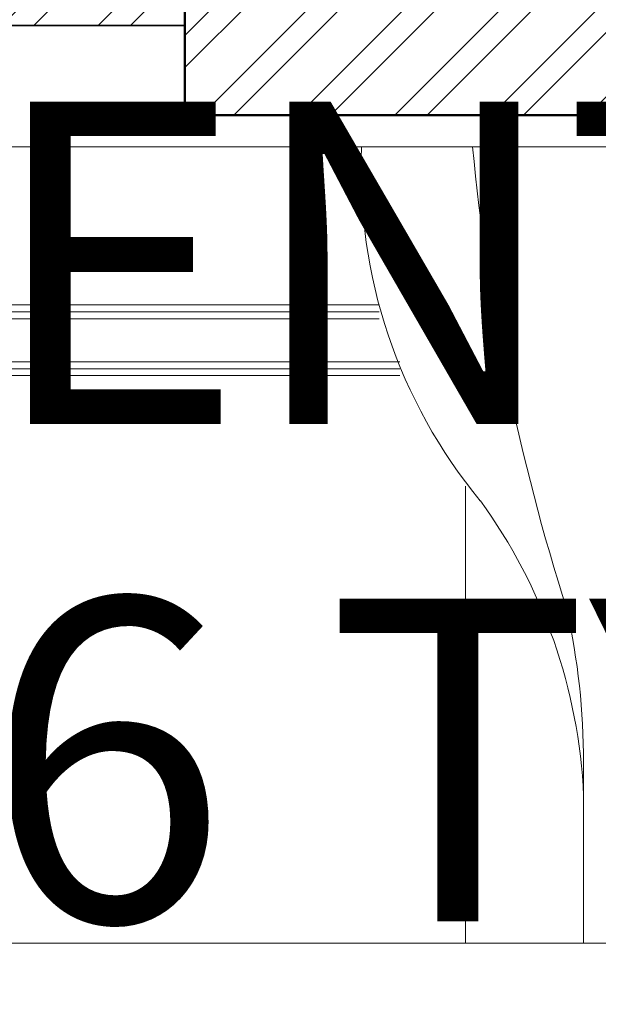
# Model space of a CAD drawing. Units: inches. Extents: x -90 to 536, y -553 to 299.
# Tile 8 of 27: x 122 to 155, y -394 to -339. Entities that reach past the tile are written whole.
import ezdxf

# ---------------------------------------------------------------- set-up
doc = ezdxf.new("R2010")
doc.units = ezdxf.units.IN
for name, color, linetype, lineweight in [('A-ANNO-DIMS', 2, 'Continuous', 18), ('A-DOOR', 4, 'Continuous', 25), ('A-WALL-PATT', 252, 'Continuous', 13), ('Furniture', 2, 'Continuous', 18), ('Inner Wall', 5, 'Continuous', 35), ('Outer Wall', 1, 'Continuous', 50)]:
    doc.layers.add(name, color=color, linetype=linetype, lineweight=lineweight)
doc.styles.get("Standard").update_dxf_attribs({"font": 'arial.ttf'})
doc.dimstyles.get("Standard").update_dxf_attribs({"dimtxt": 18, "dimasz": 12, "dimexe": 0.18, "dimexo": 0.0625, "dimgap": 0.09, "dimtad": 0, "dimtih": 1, "dimtoh": 1, "dimdec": 0, "dimzin": 0, "dimdsep": 46, "dimlunit": 3, "dimtxsty": 'Standard', "dimcen": 0.09, "dimadec": 0, "dimazin": 0, "dimtfac": 1, "dimtdec": 0, "dimtofl": 0, "dimtmove": 0, "dimatfit": 3, "dimfxl": 1, "dimtolj": 1, "dimtzin": 0, "dimarcsym": 0})

# ---------------------------------------------------------------- blocks, each defined once
blk = doc.blocks.new('A$C62731D1C')
for p, q in [((0.0963, 0.3882, 0.6857), (0.0963, 2.1408, 0.6857)), ((1.4679, 2.1408, 0.6857), (1.4679, 0.3882, 0.6857)), ((1.1569, 1.7598, 0.6857), (1.4679, 1.7598, 0.6857)), ((0.6805, 1.5566, 0.6857), (1.4679, 1.5566, 0.6857)), ((0.4664, 1.4437, 0.6857), (0.4664, 0.312, 0.6857)), ((0.4784, 1.4437, 0.6857), (0.4784, 0.312, 0.6857)), ((0.4904, 1.4437, 0.6857), (0.4904, 0.312, 0.6857)), ((0.3683, 1.4076, 0.6857), (0.3683, 0.312, 0.6857)), ((0.3803, 1.4076, 0.6857), (0.3803, 0.312, 0.6857)), ((0.3923, 1.4076, 0.6857), (0.3923, 0.312, 0.6857))]:
    blk.add_line(p, q)
for centre, radius, start, end in [((1.2552, 0.827, 0.6857), 0.9338, 92.5398, 126.0403), ((1.1565, 0.5405, 0.6857), 1.2193, 89.9814, 102.4667), ((-0.2581, 5.3461, 0.6857), 3.7939, 275.3572, 287.6665), ((0.1344, 2.2742, 0.6857), 0.8976, 267.5673, 309.5461)]:
    blk.add_arc(centre, radius, start, end)
blk = doc.blocks.new('A$C0E6D7E3D')
blk.add_blockref('A$C62731D1C', (0, 0))
blk = doc.blocks.new('DOOR-36-B')
for points in [[(37.5, 36), (37.5, 34.5), (36, 34.5), (36, 35.25), (34.5, 35.25), (34.5, 36)], [(0, 0.75), (0, 1.5), (34.5, 1.5), (34.5, 0.75)], [(37.5, 0), (37.5, 1.5), (36, 1.5), (36, 0.75), (34.5, 0.75), (34.5, 0)]]:
    blk.add_lwpolyline(points, close=True)
blk.add_arc((33.758, 1.5), 33.758, 88.7408, 180)
blk = doc.blocks.new('*D27')
at = {"layer": 'A-ANNO-DIMS', "color": 0, "lineweight": -2, "transparency": 16777216}
for p, q in [((49.132, -428.616), (49.132, -434.359)), ((86.632, -428.616), (86.632, -434.359)), ((61.132, -434.179), (74.632, -434.179)), ((86.632, -434.179), (98.632, -434.179))]:
    blk.add_line(p, q, dxfattribs=at)
at = {"layer": 'A-ANNO-DIMS', "color": 0, "transparency": 16777216}
for points in [[(61.132, -432.179), (61.132, -436.179), (49.132, -434.179)], [(74.632, -432.179), (74.632, -436.179), (86.632, -434.179)]]:
    blk.add_solid(points, dxfattribs=at)
at = {"layer": 'Defpoints', "color": 0, "transparency": 16777216}
for p in [(49.132, -428.554), (86.632, -428.554), (86.632, -434.179)]:
    blk.add_point(p, dxfattribs=at)
at = {"layer": 'A-ANNO-DIMS', "color": 0, "transparency": 16777216, "insert": (195.174, -434.179), "char_height": 18, "attachment_point": 5}
blk.add_mtext('\\A1;DOOR B 38 TYP.', dxfattribs=at)
blk = doc.blocks.new('*D28')
at = {"layer": 'A-ANNO-DIMS', "color": 0, "lineweight": -2, "transparency": 16777216}
for p, q in [((92.257, -392.554), (92.257, -380.554)), ((92.257, -380.554), (104.257, -380.554)), ((86.694, -392.554), (92.437, -392.554)), ((92.257, -416.554), (92.257, -404.554)), ((86.694, -428.554), (92.437, -428.554))]:
    blk.add_line(p, q, dxfattribs=at)
at = {"layer": 'A-ANNO-DIMS', "color": 0, "transparency": 16777216}
for points in [[(90.257, -404.554), (94.257, -404.554), (92.257, -392.554)], [(90.257, -416.554), (94.257, -416.554), (92.257, -428.554)]]:
    blk.add_solid(points, dxfattribs=at)
at = {"layer": 'Defpoints', "color": 0, "transparency": 16777216}
for p in [(86.632, -392.554), (92.257, -392.554), (86.632, -428.554)]:
    blk.add_point(p, dxfattribs=at)
at = {"layer": 'A-ANNO-DIMS', "color": 0, "transparency": 16777216, "insert": (148.15, -380.554), "char_height": 18, "attachment_point": 5}
blk.add_mtext('\\A1;36 TYP.', dxfattribs=at)
blk = doc.blocks.new('*D35')
at = {"layer": 'A-ANNO-DIMS', "color": 0, "lineweight": -2, "transparency": 16777216}
for p, q in [((233.194, -331.054), (239.837, -331.054)), ((239.657, -343.054), (239.657, -343.401)), ((239.657, -362.554), (239.657, -362.207)), ((233.194, -374.554), (239.837, -374.554))]:
    blk.add_line(p, q, dxfattribs=at)
at = {"layer": 'A-ANNO-DIMS', "color": 0, "transparency": 16777216}
for points in [[(237.657, -343.054), (241.657, -343.054), (239.657, -331.054)], [(237.657, -362.554), (241.657, -362.554), (239.657, -374.554)]]:
    blk.add_solid(points, dxfattribs=at)
at = {"layer": 'Defpoints', "color": 0, "transparency": 16777216}
for p in [(233.132, -331.054), (239.657, -331.054), (233.132, -374.554)]:
    blk.add_point(p, dxfattribs=at)
at = {"layer": 'A-ANNO-DIMS', "color": 0, "transparency": 16777216, "insert": (239.657, -352.804), "char_height": 18, "attachment_point": 5}
blk.add_mtext('\\A1;ENTRY DOOR 44 TYP.', dxfattribs=at)
blk = doc.blocks.new('*D51')
at = {"layer": 'A-ANNO-DIMS', "color": 0, "lineweight": -2, "transparency": 16777216}
for p, q in [((96.806, -393.34), (96.806, -404.606)), ((171.132, -393.34), (171.132, -404.606)), ((108.806, -404.426), (159.132, -404.426)), ((171.132, -404.426), (183.132, -404.426))]:
    blk.add_line(p, q, dxfattribs=at)
at = {"layer": 'A-ANNO-DIMS', "color": 0, "transparency": 16777216}
for points in [[(108.806, -402.426), (108.806, -406.426), (96.806, -404.426)], [(159.132, -402.426), (159.132, -406.426), (171.132, -404.426)]]:
    blk.add_solid(points, dxfattribs=at)
at = {"layer": 'Defpoints', "color": 0, "transparency": 16777216}
for p in [(96.806, -393.277), (171.132, -393.277), (171.132, -404.426)]:
    blk.add_point(p, dxfattribs=at)
at = {"layer": 'A-ANNO-DIMS', "color": 0, "transparency": 16777216, "insert": (274.99, -404.426), "char_height": 18, "attachment_point": 5}
blk.add_mtext('\\A1;SINGLE BED 74', dxfattribs=at)

msp = doc.modelspace()

# ---------------------------------------------------------------- hatches: boundary and pattern name
at = {"layer": 'A-WALL-PATT'}
h = msp.add_hatch(dxfattribs=at)
h.set_pattern_fill('ANSI32', color=256, scale=0.4)
h.set_pattern_definition([(45, (-88.8105, -603.6155), (-2.694077, 2.694077), []), (45, (-87.0145, -603.6155), (-2.694077, 2.694077), [])])
h.paths.add_polyline_path([(285.1317, 246.4462), (131.1317, 246.4462), (131.1317, 237.4462), (285.1317, 237.4462)])
h.paths.add_polyline_path([(122.1317, 237.4462), (113.1317, 237.4462), (113.1317, 152.4462), (122.1317, 152.4462), (122.1317, 166.4704)])
h.paths.add_polyline_path([(303.1317, 237.4462), (294.1317, 237.4462), (294.1317, 152.4462), (303.1317, 152.4462)])
h.paths.add_polyline_path([(47.1317, 91.9277), (38.1317, 91.9277), (38.1317, -6.5538), (77.1317, -6.5538), (77.1317, 2.4462), (70.5655, 2.4462), (47.1317, 2.4462)])
h.paths.add_polyline_path([(83.052, -61.5538), (47.1317, -61.5538), (47.1317, -24.5538), (38.1317, -24.5538), (38.1317, -70.5538), (74.052, -70.5538), (74.052, -223.5538), (38.1317, -223.5538), (38.1317, -503.5538), (92.1317, -503.5538), (92.1317, -437.5538), (191.1317, -437.5538), (191.1317, -428.5538), (83.1317, -428.5538), (83.1317, -494.5538), (47.1317, -494.5538), (47.1317, -232.5538), (83.052, -232.5538), (83.052, -70.5538)])
h.paths.add_polyline_path([(407.1317, -63.5538), (381.1317, -63.5538), (381.1317, 91.9277), (372.1317, 91.9277), (372.1317, 32.8805), (372.1317, -63.5538), (306.5745, -63.5538), (237.1317, -63.5538), (237.1317, -38.5538), (233.1317, -38.5538), (233.1317, -71.5538), (398.1317, -71.5538), (398.1317, -152.5538), (233.1317, -152.5538), (233.1317, -161.5538), (398.1317, -161.5538), (398.1317, -368.5538), (233.1317, -368.5538), (233.1317, -377.5538), (407.1317, -377.5538), (407.1317, -161.5538)])
h.paths.add_polyline_path([(261.1317, -422.5538), (252.1317, -422.5538), (252.1317, -428.5538), (233.1317, -428.5538), (233.1317, -437.5538), (261.1317, -437.5538)])
h.paths.add_polyline_path([(191.1317, -368.5538), (180.1317, -368.5538), (180.1317, -335.5538), (131.5919, -335.5538), (131.5919, -344.5538), (171.1317, -344.5538), (171.1317, -392.5538), (180.1317, -392.5538), (180.1317, -377.5538), (191.1317, -377.5538)], flags=17)
h.paths.add_polyline_path([(180.1317, -223.5538), (152.1317, -223.5538), (152.1317, -227.5538), (176.1317, -227.5538), (176.1317, -335.5538), (180.1317, -335.5538)], flags=17)
h.paths.add_polyline_path([(131.5919, -335.5538), (83.1317, -335.5538), (83.1317, -339.5538), (83.1317, -392.5538), (87.1317, -392.5538), (87.1317, -339.5538), (131.5919, -339.5538)], flags=17)
h.paths.add_polyline_path([(197.1317, 2.4462), (77.1317, 2.4462), (77.1317, -1.5538), (113.1317, -1.5538), (113.1317, -71.5538), (181.1317, -71.5538), (181.1317, -67.5538), (117.1317, -67.5538), (117.1317, -1.5538), (177.1317, -1.5538), (177.1317, -37.5538), (181.1317, -37.5538), (181.1317, -1.5538), (197.1317, -1.5538)])
h.paths.add_polyline_path([(173.1317, 138.4462), (122.1317, 138.4462), (122.1317, 134.4462), (173.1317, 134.4462)])
h.paths.add_polyline_path([(213.1317, 237.4462), (209.1317, 237.4462), (209.1317, 134.4462), (233.1317, 134.4462), (233.1317, 68.8889), (233.1317, -2.5538), (237.1317, -2.5538), (237.1317, 134.4462), (258.1317, 134.4462), (258.1317, 138.4462), (213.1317, 138.4462)])

# ---------------------------------------------------------------- linework, layer by layer
at = {"layer": 'Inner Wall'}
msp.add_line((87.1317, -339.5538), (131.5919, -339.5538), dxfattribs=at)
at = {"layer": 'Outer Wall'}
for p, q in [((131.5919, -335.5538), (131.5919, -344.5538)), ((131.5919, -344.5538), (171.1317, -344.5538))]:
    msp.add_line(p, q, dxfattribs=at)

# ---------------------------------------------------------------- block references
at = {"layer": 'A-DOOR'}
msp.add_blockref('DOOR-36-B', (139.6317, -428.5538), dxfattribs=at)
at = {"layer": 'Furniture', "xscale": 32.41097235378273, "yscale": 32.41097235378273, "zscale": 32.41097235378273, "rotation": 270}
msp.add_blockref('A$C0E6D7E3D', (96.8056, -343.2061, -22.2246), dxfattribs=at)

# ---------------------------------------------------------------- dimensions: what is measured, and where the dimension line sits
at = {"layer": 'A-ANNO-DIMS'}
for base, p1, p2, text, picture, middle in [((239.6567404714, -331.0537825705), (233.1317404714, -374.5537825705), (233.1317404714, -331.0537825705), 'ENTRY DOOR <> TYP.', '*D35', (239.6567404714, -352.8037825705)), ((92.2567, -392.5538), (86.6317, -428.5538), (86.6317, -392.5538), '<> TYP.', '*D28', (148.1496, -380.5538))]:
    dim = msp.add_linear_dim(base=base, p1=p1, p2=p2, angle=90, text=text, dimstyle='Standard', override={"dimdec": 0, "dimlfac": 1, "dimrnd": 0, "dimzin": 0, "dimdsep": 46, "dimlunit": 2}, dxfattribs=at)
    dim.commit()
    dim.dimension.update_dxf_attribs({"geometry": picture, "text_midpoint": middle})
for base, p1, p2, text, picture, middle in [((171.1317, -404.4263), (96.8056, -393.2773), (171.1317, -393.2773), 'SINGLE BED <>', '*D51', (274.9898, -404.4263)), ((86.6317404714, -434.1787825705), (49.1317404714, -428.5537825705), (86.6317404714, -428.5537825705), 'DOOR B <> TYP.', '*D27', (195.1739914946, -434.1787825705))]:
    dim = msp.add_linear_dim(base=base, p1=p1, p2=p2, text=text, dimstyle='Standard', override={"dimdec": 0, "dimlfac": 1, "dimrnd": 0, "dimzin": 0, "dimdsep": 46, "dimlunit": 2}, dxfattribs=at)
    dim.commit()
    dim.dimension.update_dxf_attribs({"geometry": picture, "text_midpoint": middle})

doc.saveas('drawing.dxf')
